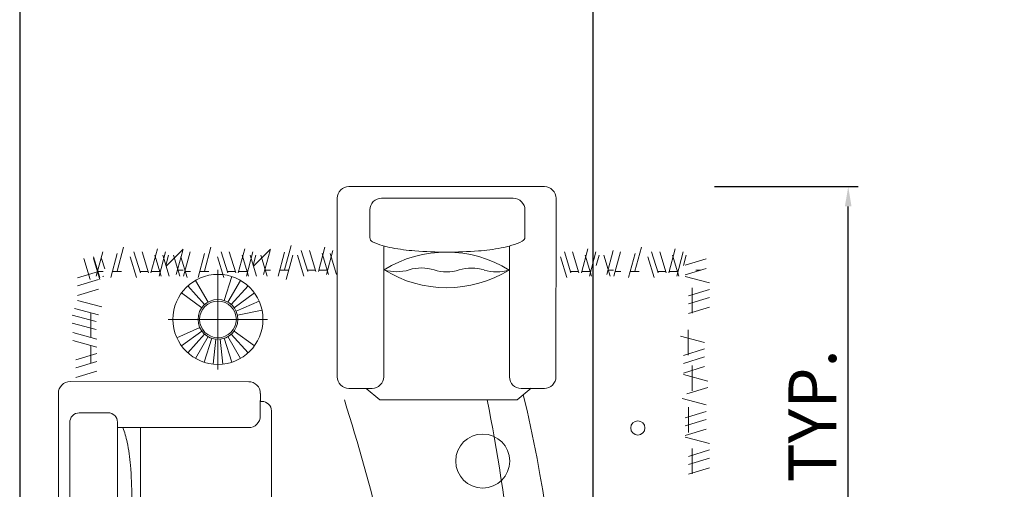
# Model space of a CAD drawing. Units: millimetres. Extents: x 20768 to 23556, y 50760 to 52704.
# Tile 12 of 36: x 20908 to 21032, y 52007 to 52066. Entities that reach past the tile are written whole.
import ezdxf

# ---------------------------------------------------------------- set-up
doc = ezdxf.new("R2010")
doc.units = ezdxf.units.MM
doc.layers.add('A-FURN', color=8, linetype='Continuous', lineweight=18)
doc.layers.add('S-ANNO-DIMS', color=2, linetype='Continuous', lineweight=18)
doc.styles.get("Standard").update_dxf_attribs({"font": 'arial.ttf'})
doc.dimstyles.new('ISO-25', dxfattribs={"dimtxt": 6, "dimasz": 2.5, "dimexe": 1.25, "dimexo": 0.625, "dimtad": 1, "dimdec": 0, "dimlunit": 3, "dimtxsty": 'Standard', "dimcen": 2.5, "dimadec": 0, "dimazin": 0, "dimtfac": 1, "dimtdec": 0, "dimtmove": 0, "dimatfit": 3, "dimfxl": 1, "dimarcsym": 0})

# ---------------------------------------------------------------- blocks, each defined once
blk = doc.blocks.new('A$C32DD204E')
for p, q in [((1063.2, 3385.6, -685.7), (1778.4, 3385.3, -685.7)), ((1020.4, 2690, -685.7), (1020.7, 3343.1, -685.7)), ((1182.2, 3343, -685.7), (1664.6, 3342.8, -685.7)), ((1820.9, 3342.8, -685.7), (1820.7, 2689.7, -685.7)), ((1139.7, 3300.5, -685.7), (1139.7, 3198.8, -685.7)), ((1707.1, 3300.3, -685.7), (1707, 3201.1, -685.7)), ((138.9, 3058.5, -685.7), (162.5, 3146.7, -685.7)), ((192.3, 3052.6, -685.7), (215.9, 3140.8, -685.7)), ((215.5, 3076.2, -685.7), (239, 3164.3, -685.7)), ((300.3, 3070.3, -685.7), (276.7, 3146.7, -685.7)), ((329.7, 3070.3, -685.7), (306.2, 3146.7, -685.7)), ((339, 3070.3, -685.7), (362.6, 3158.5, -685.7)), ((376.6, 3058.5, -685.7), (353.1, 3134.9, -685.7)), ((368.4, 3058.5, -685.7), (392, 3146.7, -685.7)), ((406, 3058.5, -685.7), (382.5, 3134.9, -685.7)), ((393.7, 3097.5, -685.7), (403.5, 3134.4, -685.7)), ((456.6, 3156.1, -685.7), (394.7, 3094.2, -685.7)), ((444.7, 3057.9, -685.7), (421.1, 3134.4, -685.7)), ((431.7, 3063.8, -685.7), (455.3, 3152, -685.7)), ((458.4, 3058.5, -685.7), (481.9, 3146.7, -685.7)), ((511.8, 3052.6, -685.7), (535.3, 3140.8, -685.7)), ((534.9, 3076.2, -685.7), (558.5, 3164.3, -685.7)), ((619.7, 3070.3, -685.7), (596.2, 3146.7, -685.7)), ((649.1, 3070.3, -685.7), (625.6, 3146.7, -685.7)), ((658.4, 3070.3, -685.7), (682, 3158.5, -685.7)), ((696.1, 3058.5, -685.7), (672.5, 3134.9, -685.7)), ((687.9, 3058.5, -685.7), (711.4, 3146.7, -685.7)), ((725.5, 3058.5, -685.7), (701.9, 3134.9, -685.7)), ((713.1, 3097.5, -685.7), (722.9, 3134.4, -685.7)), ((776, 3156.1, -685.7), (714.1, 3094.2, -685.7)), ((764.1, 3057.9, -685.7), (740.6, 3134.4, -685.7)), ((751.2, 3063.8, -685.7), (774.7, 3152, -685.7)), ((804.6, 3057.9, -685.7), (828.1, 3146.1, -685.7)), ((827.7, 3081.5, -685.7), (851.3, 3169.7, -685.7)), ((834, 3046.2, -685.7), (857.5, 3134.4, -685.7)), ((898.7, 3057.9, -685.7), (875.2, 3134.4, -685.7)), ((912.5, 3075.6, -685.7), (889, 3152, -685.7)), ((941.9, 3075.6, -685.7), (918.4, 3152, -685.7)), ((951.3, 3075.6, -685.7), (974.8, 3163.8, -685.7)), ((988.9, 3063.8, -685.7), (965.3, 3140.3, -685.7)), ((980.7, 3063.8, -685.7), (1004.2, 3152, -685.7)), ((1018.3, 3063.8, -685.7), (994.8, 3140.3, -685.7)), ((1190.7, 3168.5, -685.7), (1190.5, 2689.9, -685.7)), ((1650.7, 3168.4, -685.7), (1650.6, 2689.8, -685.7)), ((1874.9, 3070.3, -685.7), (1851.3, 3146.7, -685.7)), ((1904.3, 3070.3, -685.7), (1880.7, 3146.7, -685.7)), ((1913.6, 3070.3, -685.7), (1937.1, 3158.5, -685.7)), ((1951.2, 3058.5, -685.7), (1927.7, 3134.9, -685.7)), ((1943, 3058.5, -685.7), (1966.5, 3146.7, -685.7)), ((1968.2, 3097.5, -685.7), (1978.1, 3134.4, -685.7)), ((2019.3, 3057.9, -685.7), (1995.7, 3134.4, -685.7)), ((2006.3, 3063.8, -685.7), (2029.8, 3152, -685.7)), ((2032.9, 3058.5, -685.7), (2056.5, 3146.7, -685.7)), ((2086.3, 3052.6, -685.7), (2109.9, 3140.8, -685.7)), ((2109.5, 3076.2, -685.7), (2133, 3164.3, -685.7)), ((2194.3, 3070.3, -685.7), (2170.7, 3146.7, -685.7)), ((2223.7, 3070.3, -685.7), (2200.2, 3146.7, -685.7)), ((2233, 3070.3, -685.7), (2256.6, 3158.5, -685.7)), ((2270.6, 3058.5, -685.7), (2247.1, 3134.9, -685.7)), ((2262.4, 3058.5, -685.7), (2286, 3146.7, -685.7)), ((2287.7, 3097.5, -685.7), (2297.5, 3134.4, -685.7)), ((117, 3046.2, -685.7), (93.5, 3122.6, -685.7)), ((151.9, 3052.6, -685.7), (128.3, 3129.1, -685.7)), ((152.3, 3046.2, -685.7), (128.8, 3122.6, -685.7)), ((170, 3084.2, -685.7), (158.2, 3122.6, -685.7)), ((286.5, 3052.6, -685.7), (262.9, 3129.1, -685.7)), ((471.3, 3052.6, -685.7), (447.8, 3129.1, -685.7)), ((605.9, 3052.6, -685.7), (582.4, 3129.1, -685.7)), ((1861, 3052.6, -685.7), (1837.5, 3129.1, -685.7)), ((2180.5, 3052.6, -685.7), (2156.9, 3129.1, -685.7)), ((2370, 3121.3, -685.7), (2293.6, 3097.7, -685.7)), ((147, 3075.2, -685.7), (70.5, 3051.7, -685.7)), ((584.1, 2717, -685.7), (584.1, 3081.6, -685.7)), ((2370, 3086, -685.7), (2293.6, 3062.4, -685.7)), ((147, 3045.8, -685.7), (70.5, 3022.2, -685.7)), ((547.8, 2962.9, -685.7), (501.8, 3042.5, -685.7)), ((606.6, 2969.1, -685.7), (635, 3056.5, -685.7)), ((620.5, 2962.9, -685.7), (666.5, 3042.5, -685.7)), ((2381.8, 3033, -685.7), (2293.6, 3056.6, -685.7)), ((147, 3010.5, -685.7), (70.5, 2986.9, -685.7)), ((525.3, 2942.6, -685.7), (450.9, 2996.7, -685.7)), ((535.4, 2953.9, -685.7), (473.9, 3022.3, -685.7)), ((632.8, 2953.9, -685.7), (694.3, 3022.3, -685.7)), ((643, 2942.6, -685.7), (717.4, 2996.7, -685.7)), ((2381.8, 3009.5, -685.7), (2305.3, 2986, -685.7)), ((2319.2, 3015.1, 685.7), (2319.2, 2922.6, 685.7)), ((158.7, 2945.8, -685.7), (70.5, 2969.3, -685.7)), ((650.6, 2929.5, -685.7), (734.6, 2966.9, -685.7)), ((2381.8, 2980.1, -685.7), (2305.3, 2956.6, -685.7)), ((147, 2916.3, -685.7), (58.8, 2939.9, -685.7)), ((119.4, 2923.7, -685.7), (119.4, 2833.9, -685.7)), ((655.3, 2915, -685.7), (745.2, 2934.1, -685.7)), ((2381.8, 2944.8, -685.7), (2305.3, 2921.3, -685.7)), ((138.4, 2891.9, -685.7), (50.2, 2915.5, -685.7)), ((138.4, 2862.5, -685.7), (50.2, 2886.1, -685.7)), ((584.1, 2899.9, -685.7), (402.4, 2899.9, -685.7)), ((584.1, 2899.9, -685.7), (765.9, 2899.9, -685.7)), ((141.1, 2828.1, -685.7), (52.9, 2851.6, -685.7)), ((517.7, 2870.3, -685.7), (433.7, 2832.9, -685.7)), ((525.3, 2857.1, -685.7), (450.9, 2803.1, -685.7)), ((535.4, 2845.8, -685.7), (473.9, 2777.5, -685.7)), ((632.8, 2845.8, -685.7), (694.3, 2777.5, -685.7)), ((643, 2857.1, -685.7), (717.4, 2803.1, -685.7)), ((2304.1, 2861.1, 685.7), (2304.1, 2768.6, 685.7)), ((141.1, 2798.7, -685.7), (52.9, 2822.2, -685.7)), ((547.8, 2836.8, -685.7), (501.8, 2757.2, -685.7)), ((561.7, 2830.7, -685.7), (533.2, 2743.2, -685.7)), ((576.5, 2827.5, -685.7), (566.9, 2736.1, -685.7)), ((591.7, 2827.5, -685.7), (601.4, 2736.1, -685.7)), ((606.6, 2830.7, -685.7), (635, 2743.2, -685.7)), ((620.5, 2836.8, -685.7), (666.5, 2757.2, -685.7)), ((2364.1, 2815.4, -685.7), (2275.9, 2838.9, -685.7)), ((141.1, 2775.2, -685.7), (64.7, 2751.6, -685.7)), ((2364.1, 2791.8, -685.7), (2287.7, 2768.3, -685.7)), ((141.1, 2745.7, -685.7), (64.7, 2722.2, -685.7)), ((2364.1, 2762.4, -685.7), (2287.7, 2738.9, -685.7)), ((141.1, 2710.5, -685.7), (64.7, 2686.9, -685.7)), ((2364.1, 2727.1, -685.7), (2287.7, 2703.6, -685.7)), ((2319.2, 2731.6, 685.7), (2319.2, 2639, 685.7)), ((42.8, 2672.1, -685.7), (696.6, 2671.9, -685.7)), ((2375.9, 2674.2, -685.7), (2287.7, 2697.7, -685.7)), ((0, 755.3, -685.7), (0.2, 2629.6, -685.7)), ((1148, 2647.4, -685.7), (1062.9, 2647.5, -685.7)), ((1125.7, 2647.4, -685.7), (1176, 2605.9, -685.7)), ((1729.9, 2647.9, -685.7), (1678.7, 2605.7, -685.7)), ((1778.1, 2647.2, -685.7), (1693.1, 2647.2, -685.7)), ((2375.9, 2650.6, -685.7), (2299.4, 2627.1, -685.7)), ((738.8, 2602.8, -685.7), (738.8, 2546.5, -685.7)), ((739.1, 2598.6, -685.7), (739.1, 2629.3, -685.7)), ((739.1, 2599.7, -685.7), (745.6, 2599.7, -685.7)), ((1678.7, 2605.7, -685.7), (1176, 2605.9, -685.7)), ((2370, 2586.9, -685.7), (2281.8, 2610.4, -685.7)), ((76.8, 2558.3, -685.7), (182.2, 2558.3, -685.7)), ((779.4, 2042.5, -685.7), (779.6, 2565.6, -685.7)), ((2370, 2563.4, -685.7), (2293.6, 2539.8, -685.7)), ((2305.1, 2578.3), (2305.1, 2485.8)), ((42.1, 861.2, -685.7), (42.7, 2524.3, -685.7)), ((216, 1393.9, -685.7), (216.2, 2524.2, -685.7)), ((2370, 2534, -685.7), (2293.6, 2510.4, -685.7)), ((216.2, 2504.1, -685.7), (696.3, 2503.9, -685.7)), ((301, 1394, -685.7), (301.2, 2504.1, -685.7)), ((2370, 2498.7, -685.7), (2293.6, 2475.1, -685.7)), ((2381.8, 2445.7, -685.7), (2293.6, 2469.3, -685.7)), ((2381.8, 2422.2, -685.7), (2305.3, 2398.7, -685.7)), ((2319.2, 2427.8, 685.7), (2319.2, 2335.3, 685.7)), ((2381.8, 2392.8, -685.7), (2305.3, 2369.2, -685.7)), ((2381.8, 2357.5, -685.7), (2305.3, 2334, -685.7))]:
    blk.add_line(p, q)
at = {"elevation": -685.7}
for points in [[(163.7, 3074.4), (145.2, 3074.4)], [(230.7, 3074.4), (198.2, 3074.4)], [(328.4, 3074.4), (299, 3074.4)], [(372.7, 3074.4), (340.1, 3074.4)], [(371.7, 3074.4), (341.6, 3074.4)], [(456.5, 3079.7), (438, 3079.7)], [(483.2, 3074.4), (464.6, 3074.4)], [(550.1, 3074.4), (517.6, 3074.4)], [(647.8, 3074.4), (618.4, 3074.4)], [(692.1, 3074.4), (659.6, 3074.4)], [(691.2, 3074.4), (661, 3074.4)], [(776, 3079.7), (757.4, 3079.7)], [(842.9, 3079.7), (810.4, 3079.7)], [(940.6, 3079.7), (911.2, 3079.7)], [(984.9, 3079.7), (952.4, 3079.7)], [(984, 3079.7), (953.8, 3079.7)], [(1903, 3074.4), (1873.6, 3074.4)], [(1947.3, 3074.4), (1914.7, 3074.4)], [(1946.3, 3074.4), (1916.2, 3074.4)], [(2031.1, 3079.7), (2012.5, 3079.7)], [(2057.7, 3074.4), (2039.2, 3074.4)], [(2124.7, 3074.4), (2092.2, 3074.4)], [(2222.4, 3074.4), (2193, 3074.4)], [(2266.7, 3074.4), (2234.1, 3074.4)], [(2265.7, 3074.4), (2235.6, 3074.4)], [(2350.5, 3079.7), (2332, 3079.7)], [(119.4, 2804.5), (119.4, 2739.1)]]:
    blk.add_lwpolyline(points, dxfattribs=at)
blk.add_lwpolyline([(268.9, 2248, 0.02107), (264, 2366.2, 0.029233), (251.9, 2450.6, 0.045778), (235.8, 2504.1, 0.201615)], format="xyb", dxfattribs=at)
for centre, radius in [((584.1, 2899.9, -685.7), 164.7), ((584.1, 2899.9, -685.7), 72.8), ((584.1, 2899.9, -685.7), 67.2), ((2120.3, 2502.9, -685.7), 26), ((1552.8, 2381.6, -685.7), 98.8)]:
    blk.add_circle(centre, radius)
for centre, radius, start, end in [((1063.2, 3343.1, -685.7), 42.5, 89.9772, 179.9772), ((1778.4, 3342.8, -685.7), 42.5, 359.9772, 89.9772), ((1182.2, 3300.5, -685.7), 42.5, 89.9772, 179.9772), ((1664.6, 3300.3, -685.7), 42.5, 359.9772, 89.9772), ((1156.7, 3198.8, -685.7), 17, 179.9772, 246.2626), ((1280.5, 3480.4, -685.7), 324.6, 246.2626, 259.4626), ((1560.9, 3480.3, -685.7), 324.6, 280.4917, 294.8183), ((1690, 3201.1, -685.7), 17, 294.8183, 359.9772), ((1419.8, 2711.8, -685.7), 434.1, 58.112, 121.6703), ((1364.6, 3932.6, -685.7), 784.5, 259.4626, 265.581), ((1421.2, 4664.8, -685.7), 1518.9, 265.581, 269.9772), ((1421.2, 4664.8, -685.7), 1518.9, 269.9772, 274.3734), ((1477.2, 3932.5, -685.7), 784.5, 274.3734, 280.4917), ((1421.2, 3449.8, -685.7), 434.1, 238.112, 301.6703), ((1238.2, 3225.1, -685.7), 151.1, 252.2902, 287.4922), ((1329, 2937, -685.7), 151.1, 72.2902, 107.4922), ((1420.9, 3224.8, -685.7), 151.1, 252.2902, 287.4922), ((1511.8, 2936.6, -685.7), 151.1, 72.2902, 107.4922), ((1603.7, 3224.4, -685.7), 151.1, 252.2902, 287.4922), ((-2552.3, 2006.2, -685.7), 2911.9, 21.1287, 21.1635), ((42.8, 2629.6, -685.7), 42.5, 89.9772, 179.9772), ((696.5, 2629.3, -685.7), 42.5, 359.9772, 89.9772), ((1063, 2690, -685.7), 42.5, 179.9772, 269.9772), ((1148, 2690, -685.7), 42.5, 269.9772, 359.9772), ((1693.1, 2689.7, -685.7), 42.5, 179.9772, 269.9772), ((1778.1, 2689.7, -685.7), 42.5, 269.9772, 359.9772), ((745.5, 2565.7, -685.7), 34, 359.9772, 89.9772), ((-5717.4, 460.8, -685.7), 7095.9, 9.37507, 17.5955), ((-6034.3, 1118.6, -685.7), 7747.5, 6.78419, 11.06631), ((-3160.4, 1453.5, -685.7), 5000.5, 351.7639, 13.5399), ((77.2, 2523, -685.7), 35.2, 90.762, 182.1128), ((182.2, 2524.2, -685.7), 34, 359.9772, 89.9772), ((696.3, 2546.5, -685.7), 42.5, 269.9772, 359.9772)]:
    blk.add_arc(centre, radius, start, end)
blk = doc.blocks.new('*D191')
at = {"layer": 'Defpoints', "color": 0, "transparency": 16777216}
for p in [(20994.76, 52044.82), (21012.2, 52044.82), (20994.76, 51928.59)]:
    blk.add_point(p, dxfattribs=at)
at = {"layer": 'S-ANNO-DIMS', "color": 0, "lineweight": -2, "transparency": 16777216}
for p, q in [((20995.39, 52044.82), (21013.45, 52044.82)), ((21012.2, 51931.09), (21012.2, 52042.32)), ((20995.39, 51928.59), (21013.45, 51928.59))]:
    blk.add_line(p, q, dxfattribs=at)
at = {"layer": 'S-ANNO-DIMS', "color": 0, "transparency": 16777216}
for points in [[(21011.78, 52042.32), (21012.61, 52042.32), (21012.2, 52044.82)], [(21011.78, 51931.09), (21012.61, 51931.09), (21012.2, 51928.59)]]:
    blk.add_solid(points, dxfattribs=at)
at = {"layer": 'S-ANNO-DIMS', "color": 0, "transparency": 16777216, "insert": (21008.47, 51986.71), "char_height": 6, "attachment_point": 5, "rotation": 90}
blk.add_mtext('SOFA SET 9\'-8" TYP.', dxfattribs=at)
blk = doc.blocks.new('*D204')
at = {"layer": 'Defpoints', "color": 0, "transparency": 16777216}
for p in [(20908.14, 52080.4), (20857.64, 51900.4), (20908.14, 51900.4)]:
    blk.add_point(p, dxfattribs=at)
at = {"layer": 'S-ANNO-DIMS', "color": 0, "lineweight": -2, "transparency": 16777216}
for p, q in [((20907.51, 52080.4), (20856.39, 52080.4)), ((20857.64, 52077.9), (20857.64, 51902.9)), ((20907.51, 51900.4), (20856.39, 51900.4))]:
    blk.add_line(p, q, dxfattribs=at)
at = {"layer": 'S-ANNO-DIMS', "color": 0, "transparency": 16777216}
for points in [[(20857.22, 52077.9), (20858.06, 52077.9), (20857.64, 52080.4)], [(20857.22, 51902.9), (20858.06, 51902.9), (20857.64, 51900.4)]]:
    blk.add_solid(points, dxfattribs=at)
at = {"layer": 'S-ANNO-DIMS', "color": 0, "transparency": 16777216, "insert": (20853.95, 51990.4), "char_height": 6, "attachment_point": 5, "rotation": 90}
blk.add_mtext('15\'-0"', dxfattribs=at)
blk = doc.blocks.new('*D206')
at = {"layer": 'Defpoints', "color": 0, "transparency": 16777216}
for p in [(20908.14, 52144.9), (20980.14, 52144.9), (20980.14, 51776.4)]:
    blk.add_point(p, dxfattribs=at)
at = {"layer": 'S-ANNO-DIMS', "color": 0, "lineweight": -2, "transparency": 16777216}
for p, q in [((20908.14, 52144.27), (20908.14, 51775.15)), ((20980.14, 52144.27), (20980.14, 51775.15)), ((20910.64, 51776.4), (20977.64, 51776.4))]:
    blk.add_line(p, q, dxfattribs=at)
at = {"layer": 'S-ANNO-DIMS', "color": 0, "transparency": 16777216}
for points in [[(20910.64, 51776.81), (20910.64, 51775.98), (20908.14, 51776.4)], [(20977.64, 51776.81), (20977.64, 51775.98), (20980.14, 51776.4)]]:
    blk.add_solid(points, dxfattribs=at)
at = {"layer": 'S-ANNO-DIMS', "color": 0, "transparency": 16777216, "insert": (20944.14, 51780.09), "char_height": 6, "attachment_point": 5}
blk.add_mtext('6\'-0"', dxfattribs=at)
blk = doc.blocks.new('*D207')
at = {"layer": 'Defpoints', "color": 0, "transparency": 16777216}
for p in [(20908.14, 52080.4), (21070.14, 52080.4), (21070.14, 51776.4)]:
    blk.add_point(p, dxfattribs=at)
at = {"layer": 'S-ANNO-DIMS', "color": 0, "lineweight": -2, "transparency": 16777216}
for p, q in [((20908.14, 52079.77), (20908.14, 51775.15)), ((21070.14, 52079.77), (21070.14, 51775.15)), ((20910.64, 51776.4), (21067.64, 51776.4))]:
    blk.add_line(p, q, dxfattribs=at)
at = {"layer": 'S-ANNO-DIMS', "color": 0, "transparency": 16777216}
for points in [[(20910.64, 51776.81), (20910.64, 51775.98), (20908.14, 51776.4)], [(21067.64, 51776.81), (21067.64, 51775.98), (21070.14, 51776.4)]]:
    blk.add_solid(points, dxfattribs=at)
at = {"layer": 'S-ANNO-DIMS', "color": 0, "transparency": 16777216, "insert": (20989.14, 51780.09), "char_height": 6, "attachment_point": 5}
blk.add_mtext('13\'-6"', dxfattribs=at)

msp = doc.modelspace()

# ---------------------------------------------------------------- block references
at = {"layer": 'A-FURN', "xscale": 0.0343301531987817, "yscale": 0.0343301531987817, "zscale": 0.0343301531987817}
msp.add_blockref('A$C32DD204E', (20912.99, 51928.59, 23.54), dxfattribs=at)

# ---------------------------------------------------------------- dimensions: what is measured, and where the dimension line sits
at = {"layer": 'S-ANNO-DIMS'}
for base, p1, p2, picture, middle in [((20980.14, 51776.4), (20908.14, 52144.9), (20980.14, 52144.9), '*D206', (20944.14, 51780.09)), ((21070.14, 51776.4), (20908.14, 52080.4), (21070.14, 52080.4), '*D207', (20989.14, 51780.09))]:
    dim = msp.add_linear_dim(base=base, p1=p1, p2=p2, dimstyle='ISO-25', override={"dimdec": 1, "dimlfac": 1, "dimrnd": 0, "dimzin": 1, "dimdsep": 46, "dimlunit": 4, "dimfrac": 2}, dxfattribs=at)
    dim.commit()
    dim.dimension.update_dxf_attribs({"geometry": picture, "text_midpoint": middle})
dim = msp.add_linear_dim(base=(20857.64, 51900.4), p1=(20908.14, 52080.4), p2=(20908.14, 51900.4), angle=90, dimstyle='ISO-25', override={"dimdec": 1, "dimlfac": 1, "dimrnd": 0, "dimzin": 1, "dimdsep": 46, "dimlunit": 4, "dimfrac": 2}, dxfattribs=at)
dim.commit()
dim.dimension.update_dxf_attribs({"geometry": '*D204', "text_midpoint": (20853.95, 51990.4)})
dim = msp.add_linear_dim(base=(21012.2, 52044.82), p1=(20994.76, 51928.59), p2=(20994.76, 52044.82), angle=90, text='SOFA SET <> TYP.', dimstyle='ISO-25', override={"dimdec": 1, "dimrnd": 0, "dimzin": 1, "dimlunit": 4, "dimfrac": 2}, dxfattribs=at)
dim.commit()
dim.dimension.update_dxf_attribs({"geometry": '*D191', "text_midpoint": (21008.47, 51986.71)})

doc.saveas('drawing.dxf')
